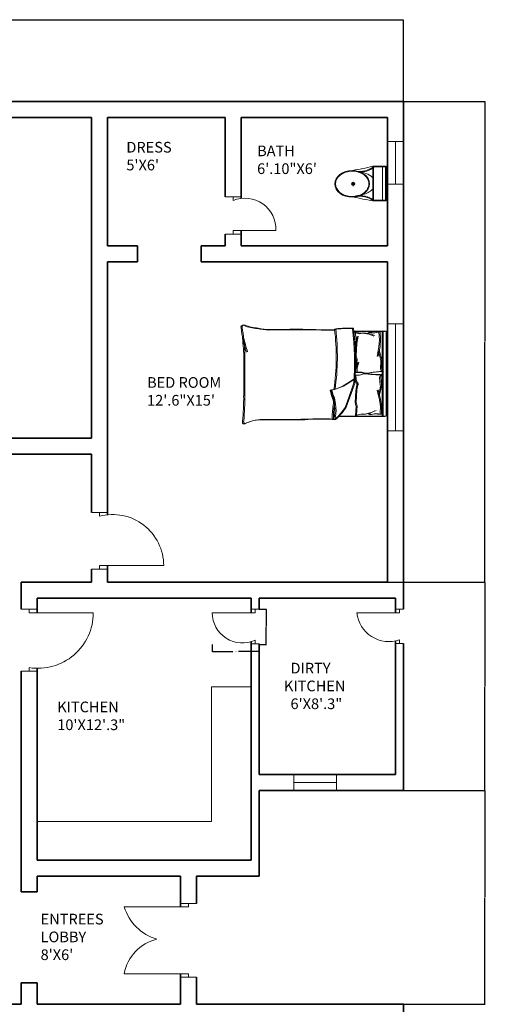
# Model space of a CAD drawing. Units: inches. Extents: x 1824 to 3509, y 619 to 2294.
# Tile 7 of 12: x 2308 to 2569, y 1115 to 1668. Entities that reach past the tile are written whole.
import ezdxf

# ---------------------------------------------------------------- set-up
doc = ezdxf.new("R2010")
doc.units = ezdxf.units.IN
for name, color, linetype, lineweight in [('A-ANNO-DIMS', 2, 'Continuous', 18), ('A-AREA-IDEN', 7, 'Continuous', 18), ('A-DOOR', 3, 'Continuous', 18), ('A-FLOR-FIXT', 9, 'Continuous', 18), ('A-FURN', 8, 'Continuous', 13), ('A-GLAZ', 4, 'Continuous', 18), ('A-WALL', 7, 'Continuous', 35)]:
    doc.layers.add(name, color=color, linetype=linetype, lineweight=lineweight)
doc.styles.get("Standard").update_dxf_attribs({"font": 'arial.ttf'})
doc.dimstyles.get("Standard").update_dxf_attribs({"dimtxt": 0.18, "dimasz": 0.18, "dimexe": 0.18, "dimexo": 0.0625, "dimgap": 0.09, "dimtad": 0, "dimtih": 1, "dimtoh": 1, "dimdec": 4, "dimzin": 0, "dimdsep": 46, "dimtxsty": 'Standard', "dimcen": 0.09, "dimadec": 0, "dimazin": 0, "dimtfac": 1, "dimtdec": 4, "dimtofl": 0, "dimtmove": 0, "dimatfit": 3, "dimfxl": 1, "dimtolj": 1, "dimtzin": 0, "dimarcsym": 0})

# ---------------------------------------------------------------- blocks, each defined once
blk = doc.blocks.new('A$C31115884')
for p, q in [((283, 498), (223, 498)), ((258, 466), (258, 523)), ((0, 200), (0, 0)), ((520, 200), (0, 200)), ((10, 190), (10, 10)), ((510, 190), (10, 190)), ((510, 10), (510, 190)), ((520, 0), (520, 200)), ((510, 54), (0, 54)), ((10, 10), (510, 10)), ((0, 0), (520, 0))]:
    blk.add_line(p, q)
blk.add_circle((256, 496), 23.6)
for centre, radius, start, end in [((2778, -205), 2807, 165.4549, 171.7133), ((-295, 403), 365, 324.2091, 9.3499), ((-295, 403), 375, 324.2091, 9.3499), ((806, 403), 365, 170.6501, 215.7909), ((3237, 905), 2807, 188.2867, 194.5451), ((384, 406), 293, 190.2774, 224.1564), ((139, 406), 293, 315.8436, 2.6563), ((806, 403), 375, 179.2036, 215.7909)]:
    blk.add_arc(centre, radius, start, end)
blk.add_ellipse((256, 510), major_axis=(0, -261), ratio=0.772727)
blk.add_open_spline([(256, 259), (263, 259), (270, 260), (288, 262), (299, 265), (320, 273), (330, 278), (350, 291), (360, 299), (378, 316), (386, 326), (402, 347), (409, 358), (421, 383), (427, 395), (436, 422), (440, 436), (445, 465), (447, 480), (448, 509), (448, 524), (445, 553), (443, 568), (436, 596), (432, 610), (422, 636), (416, 649), (402, 672), (395, 683), (379, 703), (370, 712), (351, 728), (341, 735), (321, 746), (310, 751), (289, 757), (278, 759), (256, 761), (245, 761), (223, 757), (212, 754), (191, 746), (181, 741), (161, 728), (151, 720), (133, 703), (125, 693), (110, 672), (103, 660), (90, 636), (85, 623), (76, 596), (72, 582), (67, 553), (66, 538), (64, 509), (65, 494), (68, 465), (70, 450), (77, 422), (81, 408), (91, 382), (97, 370), (111, 346), (118, 335), (135, 316), (144, 307), (162, 291), (172, 284), (193, 273), (203, 269), (225, 262), (236, 260), (250, 259), (253, 259), (256, 259)], degree=3, knots=[0, 0, 0, 0, 0.110105, 0.110105, 0.285049, 0.285049, 0.459994, 0.459994, 0.634938, 0.634938, 0.809882, 0.809882, 0.984827, 0.984827, 1.159771, 1.159771, 1.334715, 1.334715, 1.50966, 1.50966, 1.684604, 1.684604, 1.859549, 1.859549, 2.034493, 2.034493, 2.209437, 2.209437, 2.384382, 2.384382, 2.559326, 2.559326, 2.73427, 2.73427, 2.909215, 2.909215, 3.084159, 3.084159, 3.259103, 3.259103, 3.434048, 3.434048, 3.608992, 3.608992, 3.783936, 3.783936, 3.958881, 3.958881, 4.133825, 4.133825, 4.30877, 4.30877, 4.483714, 4.483714, 4.658658, 4.658658, 4.833603, 4.833603, 5.008547, 5.008547, 5.183491, 5.183491, 5.358436, 5.358436, 5.53338, 5.53338, 5.708324, 5.708324, 5.883269, 5.883269, 6.058213, 6.058213, 6.233158, 6.233158, 6.283185, 6.283185, 6.283185, 6.283185])
blk = doc.blocks.new('COUNTER-L-PLAN')
for p, q in [((120, 75.53), (97.87, 75.53)), ((97.87, 75.53), (97.87, 75.53)), ((97.87, 75.53), (97.87, 0)), ((97.87, 0), (0, 0))]:
    blk.add_line(p, q)
blk = doc.blocks.new('DOOR-BATH-E-24')
for p, q in [((9, 20.96), (0, 20.96)), ((0, 20.96), (4.5, 20.96)), ((4.5, 20.96), (4.5, 20.96)), ((4.5, 20.96), (4.5, 18.96)), ((0, 0), (9, 0)), ((4.5, 0), (4.5, 2)), ((4.5, 2), (28.5, 2)), ((5.69, 0), (4.5, 0)), ((9, 0), (5.69, 0))]:
    blk.add_line(p, q)
blk.add_arc((11.01, 2.71), 17.51, 357.6736, 111.8197)
blk = doc.blocks.new('DOOR-BED-E-36')
for p, q in [((0, 31.73), (0, 31.73)), ((0, 31.73), (9, 31.73)), ((9, 31.73), (4.5, 31.73)), ((4.5, 31.73), (4.5, 29.73)), ((9, 0), (0, 0)), ((0, 0), (4.5, 0)), ((4.5, 0), (4.5, 2)), ((4.5, 2), (40.5, 2))]:
    blk.add_line(p, q)
blk.add_arc((11.82, 2), 28.68, 0, 104.7949)
blk = doc.blocks.new('DOOR-SIDE-PAIR')
for p, q in [((36, 39.48), (0, 39.48)), ((31.5, 41.48), (40.5, 41.48)), ((40.5, 41.48), (36, 41.48)), ((36, 41.48), (36, 39.48)), ((36, 2), (0, 2)), ((31.5, 0), (40.5, 0)), ((36, 0), (36, 2)), ((40.5, 0), (36, 0))]:
    blk.add_line(p, q)
for centre, radius, start, end in [((26.04, 47.53), 27.26, 197.1823, 253.5499), ((23.91, -2.24), 24.29, 103.3084, 169.936)]:
    blk.add_arc(centre, radius, start, end)
blk = doc.blocks.new('DOOR-SERVICE-EXT-24')
for p, q in [((24, 17.22), (0, 17.22)), ((21.7, 19.22), (26.2, 19.22)), ((26.2, 19.22), (24, 19.22)), ((24, 19.22), (24, 17.22)), ((21.7, 0), (26.2, 0)), ((23.95, 0), (23.95, 2)), ((26.2, 0), (23.95, 0))]:
    blk.add_line(p, q)
blk.add_arc((18.22, 19.44), 18.36, 186.9442, 288.1646)
blk = doc.blocks.new('DOOR-SERVICE-INT-24')
for p, q in [((24, 17.35), (0, 17.35)), ((21.75, 19.35), (26.25, 19.35)), ((24, 19.35), (24, 17.35)), ((21.75, 0), (26.25, 0)), ((24, 0), (24, 2)), ((26.25, 0), (24, 0))]:
    blk.add_line(p, q)
blk.add_arc((16.91, 17.35), 16.91, 180, 294.7994)
blk = doc.blocks.new('DOOR-KITCHEN-36')
for p, q in [((0, 34.79), (9, 34.79)), ((4.5, 34.79), (4.5, 32.79)), ((4.5, 32.79), (40.5, 32.79)), ((4.5, 0), (4.5, 2)), ((0, 0), (9, 0)), ((9, 0), (4.5, 0))]:
    blk.add_line(p, q)
blk.add_arc((9.34, 32.79), 31.16, 261.0709, 0)
blk = doc.blocks.new('BED-DOUBLE-PLAN')
for p, q in [((0, 51.27), (26.61, 51.27)), ((0, 51.27), (26.61, 51.27)), ((0, 3.48), (0, 51.27)), ((0.64, 51.49), (27.25, 51.49)), ((0.64, 51.49), (27.25, 51.49)), ((1.53, 3.48), (1.53, 51.27)), ((1.53, 3.48), (1.53, 51.27)), ((2.17, 3.7), (2.17, 51.49)), ((2.17, 3.7), (2.17, 51.49)), ((2.56, 50.11), (2.46, 44.71)), ((2.56, 50.11), (2.46, 44.71)), ((2.56, 50.11), (5.77, 49.73)), ((2.56, 50.11), (5.77, 49.73)), ((3.2, 50.34), (3.1, 44.94)), ((3.2, 50.34), (3.1, 44.94)), ((3.2, 50.34), (6.41, 49.96)), ((3.2, 50.34), (6.41, 49.96)), ((5.77, 49.73), (8.34, 50.33)), ((5.77, 49.73), (8.34, 50.33)), ((6.41, 49.96), (8.98, 50.56)), ((6.41, 49.96), (8.98, 50.56)), ((11.83, 50.11), (8.26, 49.31)), ((11.83, 50.11), (8.26, 49.31)), ((8.34, 50.33), (9.38, 49.82)), ((8.34, 50.33), (9.38, 49.81)), ((12.47, 50.34), (8.9, 49.54)), ((12.47, 50.34), (8.9, 49.54)), ((8.98, 50.56), (10.02, 50.04)), ((8.98, 50.56), (10.02, 50.04)), ((13.43, 49.92), (11.83, 50.11)), ((13.43, 49.92), (11.83, 50.11)), ((14.07, 50.15), (12.47, 50.34)), ((14.07, 50.15), (12.47, 50.34)), ((16.57, 50.7), (13.43, 49.92)), ((16.57, 50.7), (13.43, 49.92)), ((17.21, 50.93), (14.07, 50.15)), ((17.21, 50.93), (14.07, 50.15)), ((16.17, 45.57), (16.57, 50.7)), ((16.17, 45.57), (16.57, 50.7)), ((16.81, 45.8), (17.21, 50.93)), ((16.81, 45.8), (17.21, 50.93)), ((27.75, 52.87), (24.5, 49.16)), ((27.75, 52.87), (24.5, 49.16)), ((28.39, 53.1), (25.13, 49.39)), ((28.39, 53.1), (25.13, 49.39)), ((29.49, 52.95), (27.75, 52.87, 3.87)), ((29.49, 52.95), (27.75, 52.87, 3.87)), ((28.36, 51.33), (27.75, 52.87)), ((28.36, 51.33), (27.75, 52.87)), ((28.06, 48.23), (28.36, 51.33)), ((28.06, 48.23), (28.36, 51.33)), ((30.13, 53.18), (28.39, 53.1, 3.87)), ((30.13, 53.18), (28.39, 53.1, 3.87)), ((29, 51.56), (28.39, 53.1)), ((29, 51.56), (28.39, 53.1)), ((28.69, 48.46), (29, 51.56)), ((28.69, 48.46), (29, 51.56)), ((2.46, 44.71), (2.54, 45.71)), ((2.46, 44.71), (2.54, 45.71)), ((2.54, 45.71), (3.07, 41.92)), ((2.54, 45.71), (3.07, 41.91)), ((3.1, 44.94), (3.18, 45.94)), ((3.1, 44.94), (3.18, 45.94)), ((3.18, 45.94), (3.71, 42.14)), ((3.18, 45.94), (3.71, 42.14)), ((8.26, 49.31), (5.58, 48.13)), ((8.26, 49.31), (5.58, 48.13)), ((8.9, 49.54), (6.22, 48.36)), ((8.9, 49.54), (6.22, 48.36)), ((16.73, 43.61), (16.17, 45.57)), ((16.73, 43.61), (16.17, 45.57)), ((17.37, 43.84), (16.81, 45.8)), ((17.37, 43.83), (16.81, 45.8)), ((22.33, 46.22), (20.32, 40.64)), ((22.33, 46.22), (20.32, 40.64)), ((22.97, 46.45), (20.96, 40.87)), ((22.97, 46.45), (20.96, 40.87)), ((24.5, 49.16), (22.33, 46.22)), ((24.5, 49.16), (22.33, 46.22)), ((25.13, 49.39), (22.97, 46.45)), ((25.13, 49.39), (22.97, 46.45)), ((28.36, 44.36), (28.06, 48.23)), ((28.36, 44.36), (28.06, 48.23)), ((28.83, 40.95), (28.36, 44.36)), ((28.83, 40.95), (28.36, 44.36)), ((29, 44.59), (28.69, 48.46)), ((29, 44.59), (28.69, 48.46)), ((29.47, 41.18), (29, 44.59)), ((29.47, 41.18), (29, 44.59)), ((3.07, 41.92), (4.42, 36.5)), ((3.07, 41.91), (4.42, 36.5)), ((3.67, 39.2), (3.08, 37.14)), ((3.67, 39.2), (3.08, 37.14)), ((3.71, 42.14), (5.06, 36.72)), ((3.71, 42.14), (5.06, 36.72)), ((4.31, 39.43), (3.72, 37.36)), ((4.31, 39.43), (3.72, 37.36)), ((16.3, 36.6), (16.73, 43.61)), ((16.3, 36.6), (16.73, 43.61)), ((16.93, 36.83), (17.37, 43.84)), ((16.93, 36.82), (17.37, 43.83)), ((20.32, 40.64), (17.38, 32.31)), ((20.32, 40.64), (17.38, 32.31)), ((20.96, 40.87), (18.02, 32.54)), ((20.96, 40.87), (18.02, 32.53)), ((29.76, 38.94), (28.83, 40.95)), ((29.76, 38.94), (28.83, 40.95)), ((30.4, 39.17), (29.47, 41.18)), ((30.4, 39.17), (29.47, 41.18)), ((30.38, 36.46), (29.76, 38.94)), ((30.38, 36.46), (29.76, 38.94)), ((31.02, 36.69), (30.4, 39.17)), ((31.02, 36.69), (30.4, 39.17)), ((79.24, 15.06), (79.24, 39.68)), ((79.24, 15.06), (79.24, 39.68)), ((79.88, 15.29), (79.88, 39.91)), ((79.88, 15.29), (79.88, 39.91)), ((3.08, 37.14), (2.54, 34.21)), ((3.08, 37.14), (2.54, 34.21)), ((2.54, 34.21), (2.56, 33.88)), ((2.54, 34.21), (2.56, 33.88)), ((2.56, 33.88), (2.98, 29.46)), ((2.56, 33.88), (2.98, 29.46)), ((3.72, 37.36), (3.18, 34.43)), ((3.72, 37.36), (3.18, 34.43)), ((3.18, 34.43), (3.2, 34.11)), ((3.18, 34.43), (3.2, 34.11)), ((3.2, 34.11), (3.62, 29.68)), ((3.2, 34.11), (3.62, 29.68)), ((16.74, 30.75), (15.45, 33.82)), ((16.74, 30.75), (15.45, 33.82)), ((15.63, 32.56), (16.3, 36.6)), ((15.63, 32.56), (16.3, 36.6)), ((17.38, 30.98), (16.09, 34.05)), ((17.38, 30.98), (16.09, 34.05)), ((16.27, 32.79), (16.93, 36.83)), ((16.27, 32.79), (16.93, 36.82)), ((17.38, 30.26), (23.88, 34.45)), ((17.38, 30.26), (23.88, 34.45)), ((18.02, 30.49), (24.52, 34.68)), ((18.02, 30.49), (24.52, 34.68)), ((23.88, 34.45), (28.36, 36.15)), ((23.88, 34.45), (28.36, 36.15)), ((24.52, 34.68), (29, 36.38)), ((24.52, 34.68), (29, 36.38)), ((28.36, 36.15), (30.38, 36.46)), ((28.36, 36.15), (30.38, 36.46)), ((29, 36.38), (31.02, 36.69)), ((29, 36.38), (31.02, 36.69)), ((2.98, 29.46), (2.49, 27.98)), ((2.98, 29.46), (2.49, 27.98)), ((2.49, 27.98), (7.87, 27.73)), ((2.49, 27.98), (7.87, 27.73)), ((3.62, 29.68), (3.13, 28.21)), ((3.62, 29.68), (3.13, 28.21)), ((3.13, 28.21), (8.51, 27.96)), ((3.13, 28.21), (8.51, 27.96)), ((7.87, 27.73), (11.08, 27.36)), ((7.87, 27.73), (11.08, 27.36)), ((8.51, 27.96), (11.72, 27.58)), ((8.51, 27.96), (11.72, 27.58)), ((11.72, 27.58), (13.02, 27.67)), ((11.72, 27.58), (13.02, 27.66)), ((12.38, 27.44), (14.22, 28.13)), ((12.38, 27.44), (14.22, 28.13)), ((13.02, 27.67), (14.86, 28.36)), ((13.02, 27.66), (14.86, 28.36)), ((14.22, 28.13), (16.89, 28.3)), ((14.22, 28.13), (16.89, 28.3)), ((14.86, 28.36), (17.53, 28.53)), ((14.86, 28.36), (17.53, 28.53)), ((16.89, 28.3), (16.74, 30.75)), ((16.89, 28.3), (16.74, 30.75)), ((17.53, 28.53), (17.38, 30.98)), ((17.53, 28.53), (17.38, 30.98)), ((1.87, 25.98), (7.22, 26.56)), ((1.87, 25.98), (7.22, 26.56)), ((2.45, 24.54), (1.87, 25.98)), ((2.45, 24.54), (1.87, 25.98)), ((2.3, 20.09), (2.45, 24.54)), ((2.3, 20.09), (2.45, 24.54)), ((2.51, 26.21), (7.86, 26.79)), ((2.51, 26.21), (7.86, 26.79)), ((3.09, 24.77), (2.51, 26.21)), ((3.09, 24.77), (2.51, 26.21)), ((2.94, 20.32), (3.09, 24.77)), ((2.94, 20.32), (3.09, 24.77)), ((7.22, 26.56), (10.4, 27.14)), ((7.22, 26.56), (10.4, 27.14)), ((7.86, 26.79), (11.04, 27.37)), ((7.86, 26.79), (11.04, 27.37)), ((10.4, 27.14), (11.7, 27.14)), ((10.4, 27.14), (11.7, 27.14)), ((11.04, 27.37), (12.34, 27.37)), ((11.04, 27.37), (12.34, 27.37)), ((11.08, 27.36), (12.38, 27.44)), ((11.08, 27.36), (12.38, 27.44)), ((11.7, 27.14), (13.58, 26.56)), ((11.7, 27.14), (13.58, 26.56)), ((12.34, 27.37), (14.22, 26.79)), ((12.34, 27.37), (14.22, 26.79)), ((13.58, 26.56), (16.26, 26.56)), ((13.58, 26.56), (16.26, 26.56)), ((14.22, 26.79), (16.9, 26.79)), ((14.22, 26.79), (16.9, 26.79)), ((16.26, 24.1), (15.17, 20.96)), ((16.26, 24.1), (15.17, 20.96)), ((16.9, 24.33), (15.81, 21.19)), ((16.9, 24.33), (15.81, 21.19)), ((16.17, 19.38), (16.57, 24.52)), ((16.17, 19.38), (16.57, 24.52)), ((16.26, 26.56), (16.26, 24.1)), ((16.26, 26.56), (16.26, 24.1)), ((16.81, 19.61), (17.21, 24.74)), ((16.81, 19.61), (17.21, 24.74)), ((16.9, 26.79), (16.9, 24.33)), ((16.9, 26.79), (16.9, 24.33)), ((2.3, 19.77), (2.3, 20.09)), ((2.3, 19.77), (2.3, 20.09)), ((3.03, 16.88), (2.3, 19.77)), ((3.03, 16.88), (2.3, 19.77)), ((2.94, 20), (2.94, 20.32)), ((2.94, 20), (2.94, 20.32)), ((3.67, 17.11), (2.94, 20)), ((3.67, 17.11), (2.94, 20)), ((3.75, 14.86), (3.03, 16.88)), ((3.75, 14.86), (3.03, 16.88)), ((3.32, 12.11), (4.33, 17.6)), ((3.32, 12.11), (4.33, 17.6)), ((4.39, 15.08), (3.67, 17.11)), ((4.39, 15.08), (3.67, 17.11)), ((3.96, 12.34), (4.97, 17.83)), ((3.96, 12.34), (4.97, 17.83)), ((16.73, 17.42), (16.17, 19.38)), ((16.73, 17.42), (16.17, 19.38)), ((16.3, 10.41), (16.73, 17.42)), ((16.3, 10.41), (16.73, 17.42)), ((17.37, 17.65), (16.81, 19.61)), ((17.37, 17.65), (16.81, 19.61)), ((16.93, 10.64), (17.37, 17.65)), ((16.93, 10.64), (17.37, 17.65)), ((3.03, 8.29), (3.32, 12.11)), ((3.03, 8.29), (3.32, 12.11)), ((3.67, 8.51), (3.96, 12.34)), ((3.67, 8.51), (3.96, 12.34)), ((3.01, 8.18), (3.03, 8.29)), ((3.01, 8.18), (3.03, 8.29)), ((3.34, 3.9), (3.01, 8.18)), ((3.34, 3.9), (3.01, 8.18)), ((3.65, 8.41), (3.67, 8.51)), ((3.65, 8.41), (3.67, 8.51)), ((3.98, 4.13), (3.65, 8.41)), ((3.98, 4.13), (3.65, 8.41)), ((8.95, 5.05), (6.21, 6.06)), ((8.95, 5.05), (6.21, 6.06)), ((9.59, 5.28), (6.85, 6.29)), ((9.59, 5.28), (6.85, 6.29)), ((15.63, 6.38), (16.3, 10.41)), ((15.63, 6.38), (16.3, 10.41)), ((16.27, 6.61), (16.93, 10.64)), ((16.27, 6.61), (16.93, 10.64)), ((16.3, 10.41), (16.62, 9.28)), ((16.3, 10.41), (16.62, 9.28)), ((16.62, 9.28), (17.34, 4.18)), ((16.62, 9.28), (17.34, 4.18)), ((16.93, 10.64), (17.26, 9.51)), ((16.93, 10.64), (17.26, 9.51)), ((17.26, 9.51), (17.98, 4.41)), ((17.26, 9.51), (17.98, 4.41)), ((18.11, 3.48), (0, 3.48)), ((18.11, 3.48), (0, 3.48)), ((18.75, 3.7), (0.64, 3.7)), ((18.75, 3.7), (0.64, 3.7)), ((3.32, 3.9), (6.5, 4.47)), ((3.32, 3.9), (6.5, 4.47)), ((3.96, 4.12), (7.14, 4.7)), ((3.96, 4.12), (7.14, 4.7)), ((6.5, 4.47), (9.1, 4.04)), ((6.5, 4.47), (9.1, 4.04)), ((7.14, 4.7), (9.74, 4.27)), ((7.14, 4.7), (9.74, 4.27)), ((12.57, 4.47), (8.95, 5.05)), ((12.57, 4.47), (8.95, 5.05)), ((9.1, 4.04), (10.11, 4.62)), ((9.1, 4.04), (10.11, 4.62)), ((13.21, 4.7), (9.59, 5.28)), ((13.21, 4.7), (9.59, 5.28)), ((9.74, 4.27), (10.75, 4.85)), ((9.74, 4.27), (10.75, 4.85)), ((14.16, 4.76), (12.57, 4.47)), ((14.16, 4.76), (12.57, 4.47)), ((14.8, 4.99), (13.21, 4.7)), ((14.8, 4.99), (13.21, 4.7)), ((17.34, 4.18), (14.16, 4.76)), ((17.34, 4.18), (14.16, 4.76)), ((17.98, 4.41), (14.8, 4.99)), ((17.98, 4.41), (14.8, 4.99))]:
    blk.add_line(p, q)
for centre, radius, start, end in [((68.67, 76.16), 23.07, 267.4714, 296.4681), ((68.67, 76.16), 23.07, 267.4714, 296.4681), ((69.31, 76.39), 23.07, 267.4714, 296.4681), ((69.31, 76.39), 23.07, 267.4714, 296.4681), ((78.87, 54.41), 1.1, 332.6588, 86.02), ((78.87, 54.41), 1.1, 332.6588, 86.02), ((79.51, 54.64), 1.1, 332.6588, 86.02), ((79.51, 54.64), 1.1, 332.6588, 86.02), ((-6.66, 51.33), 36.18, 349.8763, 2.5657), ((-6.66, 51.33), 36.18, 349.8763, 2.5657), ((36.32, 182.27), 129.5, 266.9791, 273.8365), ((36.32, 182.27), 129.5, 266.9791, 273.8365), ((-6.02, 51.56), 36.18, 349.8763, 2.5657), ((-6.02, 51.56), 36.18, 349.8763, 2.5657), ((36.95, 182.49), 129.5, 266.9791, 273.8365), ((36.95, 182.49), 129.5, 266.9791, 273.8365), ((67.82, -4508.74), 4561.86, 90.00217, 90.28689), ((67.82, -4508.74), 4561.86, 90.00217, 90.28689), ((68.46, -4508.51), 4561.86, 90.00217, 90.28689), ((68.46, -4508.51), 4561.86, 90.00217, 90.28689), ((212.28, 41.15), 133.04, 174.4998, 180.6351), ((212.28, 41.15), 133.04, 174.4998, 180.6351), ((212.92, 41.38), 133.04, 174.4998, 180.6351), ((212.92, 41.38), 133.04, 174.4998, 180.6351), ((35.07, 43.74), 6.22, 168.6608, 203.7384), ((35.07, 43.74), 6.22, 168.6608, 203.7384), ((35.71, 43.97), 6.22, 168.6608, 203.7384), ((35.71, 43.97), 6.22, 168.6608, 203.7384), ((1.48, 31.15), 29.65, 10.6617, 19.8806), ((1.48, 31.15), 29.65, 10.6617, 19.8806), ((2.12, 31.38), 29.65, 10.6617, 19.8806), ((2.12, 31.38), 29.65, 10.6617, 19.8806), ((156.32, 17.76), 129.02, 171.7845, 186.9006), ((156.32, 17.76), 129.02, 171.7845, 186.9006), ((156.96, 17.98), 129.02, 171.7845, 186.9006), ((156.96, 17.98), 129.02, 171.7845, 186.9006), ((30.44, 36.64), 0.185, 250.2464, 1.1377), ((30.44, 36.64), 0.185, 250.2464, 1.1377), ((31.08, 36.87), 0.185, 250.2464, 1.1377), ((31.08, 36.87), 0.185, 250.2464, 1.1377), ((182.05, 21.36), 164.97, 176.0865, 186.7821), ((182.05, 21.36), 164.97, 176.0865, 186.7821), ((182.69, 21.59), 164.97, 176.0865, 186.7821), ((182.69, 21.59), 164.97, 176.0865, 186.7821), ((-23.71, -17.22), 106.46, 13.3832, 17.7053), ((-23.71, -17.22), 106.46, 13.3832, 17.7053), ((-23.07, -16.99), 106.46, 13.3832, 17.7053), ((-23.07, -16.99), 106.46, 13.3832, 17.7053), ((200.84, 21.43), 121.76, 182.9958, 189.4091), ((200.84, 21.43), 121.76, 182.9958, 189.4091), ((201.48, 21.66), 121.76, 182.9958, 189.4091), ((201.48, 21.66), 121.76, 182.9958, 189.4091), ((20.1, 85.16), 83.31, 268.7218, 275.604), ((20.1, 85.16), 83.31, 268.7218, 275.604), ((20.74, 85.39), 83.31, 268.7218, 275.604), ((20.74, 85.39), 83.31, 268.7218, 275.604), ((31.17, -167.31), 170.11, 88.4762, 91.0082), ((31.17, -167.31), 170.11, 88.4762, 91.0082), ((31.81, -167.08), 170.11, 88.4762, 91.0082), ((31.81, -167.08), 170.11, 88.4762, 91.0082), ((50.61, 484.82), 482.31, 268.2277, 271.7185), ((50.61, 484.82), 482.31, 268.2277, 271.7185), ((51.25, 485.05), 482.31, 268.2277, 271.7185), ((51.25, 485.05), 482.31, 268.2277, 271.7185), ((64.52, -26.9), 29.63, 76.0648, 88.9113), ((64.52, -26.9), 29.63, 76.0648, 88.9113), ((65.15, -26.67), 29.63, 76.0648, 88.9113), ((65.15, -26.67), 29.63, 76.0648, 88.9113), ((70.28, -21.66), 23.56, 67.9751, 86.652), ((70.28, -21.66), 23.56, 67.9751, 86.652), ((70.91, -21.43), 23.56, 67.9751, 86.652), ((70.91, -21.43), 23.56, 67.9751, 86.652), ((79.72, 1.09), 1.09, 236.1736, 23.4781), ((79.72, 1.09), 1.09, 236.1736, 23.4781), ((80.36, 1.32), 1.09, 236.1736, 23.4781), ((80.36, 1.32), 1.09, 236.1736, 23.4781)]:
    blk.add_arc(centre, radius, start, end)
blk = doc.blocks.new('WIN-24')
for p, q in [((0, 0), (0, 9)), ((0, 9), (0, 4.5)), ((24, 0), (24, 9)), ((0, 4.5), (24, 4.5)), ((24, 4.5), (24, 0))]:
    blk.add_line(p, q)
blk = doc.blocks.new('WIN-60')
for p, q in [((0, 9), (0, 0)), ((60, 4.5), (60, 9)), ((60, 9), (60, 0)), ((0, 0), (0, 4.5)), ((0, 4.5), (60, 4.5))]:
    blk.add_line(p, q)
blk = doc.blocks.new('*D70')
at = {"layer": 'A-ANNO-DIMS', "color": 0, "lineweight": -2, "transparency": 16777216}
for p, q in [((2415.84, 1317.1), (2415.84, 1313.04)), ((2442.09, 1317.1), (2442.09, 1313.04)), ((2416.02, 1313.22), (2427.44, 1313.22)), ((2441.91, 1313.22), (2430.49, 1313.22))]:
    blk.add_line(p, q, dxfattribs=at)
at = {"layer": 'A-ANNO-DIMS', "color": 0, "transparency": 16777216}
for points in [[(2416.02, 1313.25), (2416.02, 1313.19), (2415.84, 1313.22)], [(2441.91, 1313.25), (2441.91, 1313.19), (2442.09, 1313.22)]]:
    blk.add_solid(points, dxfattribs=at)
at = {"layer": 'Defpoints', "color": 0, "transparency": 16777216}
for p in [(2415.84, 1317.16), (2442.09, 1317.16), (2442.09, 1313.22)]:
    blk.add_point(p, dxfattribs=at)
at = {"layer": 'A-ANNO-DIMS', "color": 0, "transparency": 16777216, "insert": (2428.96, 1313.22), "char_height": 0.18, "attachment_point": 5}
blk.add_mtext('\\A1;SERVICE DOOR 26 TYP.', dxfattribs=at)
blk = doc.blocks.new('*D71')
at = {"layer": 'A-ANNO-DIMS', "color": 0, "lineweight": -2, "transparency": 16777216}
for p, q in [((2442.15, 1336.93), (2446.21, 1336.93)), ((2446.03, 1336.75), (2446.03, 1327.23)), ((2446.03, 1317.34), (2446.03, 1326.86)), ((2442.15, 1317.16), (2446.21, 1317.16))]:
    blk.add_line(p, q, dxfattribs=at)
at = {"layer": 'A-ANNO-DIMS', "color": 0, "transparency": 16777216}
for points in [[(2446, 1336.75), (2446.06, 1336.75), (2446.03, 1336.93)], [(2446, 1317.34), (2446.06, 1317.34), (2446.03, 1317.16)]]:
    blk.add_solid(points, dxfattribs=at)
at = {"layer": 'Defpoints', "color": 0, "transparency": 16777216}
for p in [(2442.09, 1336.93), (2446.03, 1336.93), (2442.09, 1317.16)]:
    blk.add_point(p, dxfattribs=at)
at = {"layer": 'A-ANNO-DIMS', "color": 0, "transparency": 16777216, "insert": (2446.03, 1327.05), "char_height": 0.18, "attachment_point": 5}
blk.add_mtext('\\A1;20 TYP.', dxfattribs=at)
blk = doc.blocks.new('*D94')
at = {"layer": 'A-ANNO-DIMS', "color": 0, "lineweight": -2, "transparency": 16777216}
for p, q in [((1949.09, 1049.16), (1949.09, 1668.03)), ((1949.27, 1667.85), (2235.8, 1667.85)), ((2522.91, 1667.85), (2236.38, 1667.85)), ((2523.09, 1622.16), (2523.09, 1668.03))]:
    blk.add_line(p, q, dxfattribs=at)
at = {"layer": 'A-ANNO-DIMS', "color": 0, "transparency": 16777216}
for points in [[(1949.27, 1667.88), (1949.27, 1667.82), (1949.09, 1667.85)], [(2522.91, 1667.88), (2522.91, 1667.82), (2523.09, 1667.85)]]:
    blk.add_solid(points, dxfattribs=at)
at = {"layer": 'Defpoints', "color": 0, "transparency": 16777216}
for p in [(2523.09, 1667.85), (2523.09, 1622.1), (1949.09, 1049.1)]:
    blk.add_point(p, dxfattribs=at)
at = {"layer": 'A-ANNO-DIMS', "color": 0, "transparency": 16777216, "insert": (2236.09, 1667.85), "char_height": 0.18, "attachment_point": 5}
blk.add_mtext('\\A1;574', dxfattribs=at)
blk = doc.blocks.new('*D98')
at = {"layer": 'A-ANNO-DIMS', "color": 0, "lineweight": -2, "transparency": 16777216}
for p, q in [((2523.15, 1235.1), (2569.02, 1235.1)), ((2568.84, 1234.92), (2568.84, 1175.28)), ((2568.84, 1115.28), (2568.84, 1174.92)), ((2523.15, 1115.1), (2569.02, 1115.1))]:
    blk.add_line(p, q, dxfattribs=at)
at = {"layer": 'A-ANNO-DIMS', "color": 0, "transparency": 16777216}
for points in [[(2568.81, 1234.92), (2568.87, 1234.92), (2568.84, 1235.1)], [(2568.81, 1115.28), (2568.87, 1115.28), (2568.84, 1115.1)]]:
    blk.add_solid(points, dxfattribs=at)
at = {"layer": 'Defpoints', "color": 0, "transparency": 16777216}
for p in [(2523.09, 1235.1), (2568.84, 1235.1), (2523.09, 1115.1)]:
    blk.add_point(p, dxfattribs=at)
at = {"layer": 'A-ANNO-DIMS', "color": 0, "transparency": 16777216, "insert": (2568.84, 1175.1), "char_height": 0.18, "attachment_point": 5}
blk.add_mtext('\\A1;120', dxfattribs=at)
blk = doc.blocks.new('*D99')
at = {"layer": 'A-ANNO-DIMS', "color": 0, "lineweight": -2, "transparency": 16777216}
for p, q in [((2514.15, 1352.1), (2569.02, 1352.1)), ((2568.84, 1351.92), (2568.84, 1293.78)), ((2568.84, 1235.28), (2568.84, 1293.42)), ((2523.15, 1235.1), (2569.02, 1235.1))]:
    blk.add_line(p, q, dxfattribs=at)
at = {"layer": 'A-ANNO-DIMS', "color": 0, "transparency": 16777216}
for points in [[(2568.81, 1351.92), (2568.87, 1351.92), (2568.84, 1352.1)], [(2568.81, 1235.28), (2568.87, 1235.28), (2568.84, 1235.1)]]:
    blk.add_solid(points, dxfattribs=at)
at = {"layer": 'Defpoints', "color": 0, "transparency": 16777216}
for p in [(2514.09, 1352.1), (2568.84, 1352.1), (2523.09, 1235.1)]:
    blk.add_point(p, dxfattribs=at)
at = {"layer": 'A-ANNO-DIMS', "color": 0, "transparency": 16777216, "insert": (2568.84, 1293.6), "char_height": 0.18, "attachment_point": 5}
blk.add_mtext('\\A1;117', dxfattribs=at)
blk = doc.blocks.new('*D100')
at = {"layer": 'A-ANNO-DIMS', "color": 0, "lineweight": -2, "transparency": 16777216}
for p, q in [((2523.15, 1622.1), (2569.02, 1622.1)), ((2568.84, 1621.92), (2568.84, 1487.28)), ((2568.84, 1352.28), (2568.84, 1486.92)), ((2514.15, 1352.1), (2569.02, 1352.1))]:
    blk.add_line(p, q, dxfattribs=at)
at = {"layer": 'A-ANNO-DIMS', "color": 0, "transparency": 16777216}
for points in [[(2568.81, 1621.92), (2568.87, 1621.92), (2568.84, 1622.1)], [(2568.81, 1352.28), (2568.87, 1352.28), (2568.84, 1352.1)]]:
    blk.add_solid(points, dxfattribs=at)
at = {"layer": 'Defpoints', "color": 0, "transparency": 16777216}
for p in [(2523.09, 1622.1), (2568.84, 1622.1), (2514.09, 1352.1)]:
    blk.add_point(p, dxfattribs=at)
at = {"layer": 'A-ANNO-DIMS', "color": 0, "transparency": 16777216, "insert": (2568.84, 1487.1), "char_height": 0.18, "attachment_point": 5}
blk.add_mtext('\\A1;270', dxfattribs=at)

msp = doc.modelspace()

# ---------------------------------------------------------------- linework, layer by layer
at = {"layer": 'A-GLAZ'}
msp.add_line((2523.0899, 1599.654), (2523.0899, 1599.654), dxfattribs=at)
at = {"layer": 'A-WALL'}
for p, q in [((2006.0899, 1622.1012), (2523.0899, 1622.1012)), ((2523.0899, 1622.1012), (2523.0899, 1336.9292)), ((2192.0899, 1613.1012), (2348.0899, 1613.1012)), ((2348.0899, 1613.1012), (2348.0899, 1433.1012)), ((2357.0899, 1613.1012), (2357.0899, 1541.1012)), ((2357.0899, 1613.1012), (2423.0899, 1613.1012)), ((2423.0899, 1613.1012), (2423.0899, 1568.5597)), ((2432.0899, 1613.1012), (2432.0899, 1567.6985)), ((2432.0899, 1613.1012), (2514.0899, 1613.1012)), ((2514.0899, 1613.1012), (2514.0899, 1541.1012)), ((2432.0899, 1549.5961), (2432.0899, 1541.1012)), ((2423.0899, 1547.5961), (2423.0899, 1541.1012)), ((2357.0899, 1541.1012), (2373.9772, 1541.1012)), ((2373.9772, 1541.1012), (2373.9772, 1532.1012)), ((2409.6371, 1541.1012), (2409.6371, 1532.1012)), ((2409.6371, 1541.1012), (2423.0899, 1541.1012)), ((2432.0899, 1541.1012), (2514.0899, 1541.1012)), ((2357.0899, 1532.1012), (2373.9772, 1532.1012)), ((2357.0899, 1532.1012), (2357.0899, 1390.0103)), ((2409.6371, 1532.1012), (2514.0899, 1532.1012)), ((2514.0899, 1532.1012), (2514.0899, 1352.1012)), ((2235.3516, 1433.1012), (2348.0899, 1433.1012)), ((2237.6334, 1424.1012), (2348.0899, 1424.1012)), ((2348.0899, 1424.1012), (2348.0899, 1391.1988)), ((2357.0899, 1361.4725), (2357.0899, 1352.1012)), ((2348.0899, 1359.4725), (2348.0899, 1352.1012)), ((2308.5899, 1343.1012), (2308.5899, 1352.1012)), ((2308.5899, 1352.1012), (2348.0899, 1352.1012)), ((2357.0899, 1352.1012), (2514.0899, 1352.1012)), ((2308.5899, 1343.1012), (2308.5899, 1336.9292)), ((2317.5899, 1343.1012), (2317.5899, 1334.9292)), ((2357.0899, 1343.1012), (2317.5899, 1343.1012)), ((2357.0899, 1343.1012), (2437.5899, 1343.1012)), ((2437.5899, 1343.1012), (2437.5899, 1334.9292)), ((2442.0899, 1343.1012), (2442.0899, 1336.9292)), ((2442.0899, 1343.1012), (2514.0899, 1343.1012)), ((2514.0899, 1343.1012), (2518.5899, 1343.1012)), ((2518.5899, 1343.1012), (2518.5899, 1334.9292)), ((2437.5899, 1318.7293), (2437.5899, 1196.1012)), ((2442.0899, 1317.5804), (2442.0899, 1244.1012)), ((2518.5899, 1319.1219), (2518.5899, 1244.1012)), ((2523.0899, 1317.7052), (2523.0899, 1235.1012)), ((2308.5899, 1302.1437), (2308.5899, 1178.3005)), ((2317.5899, 1303.7679), (2317.5899, 1196.1012)), ((2442.0899, 1244.1012), (2518.5899, 1244.1012)), ((2442.0899, 1235.1012), (2514.0899, 1235.1012)), ((2442.0899, 1235.1012), (2442.0899, 1187.1012)), ((2514.0899, 1235.1012), (2523.0899, 1235.1012)), ((2357.0899, 1196.1012), (2317.5899, 1196.1012)), ((2357.0899, 1196.1012), (2437.5899, 1196.1012)), ((2357.0899, 1187.1012), (2317.5899, 1187.1012)), ((2317.5899, 1187.1012), (2317.5899, 1178.3005)), ((2357.0899, 1187.1012), (2397.9516, 1187.1012)), ((2397.9516, 1187.1012), (2397.9516, 1169.754)), ((2406.9516, 1171.754), (2406.9516, 1187.1012)), ((2406.9516, 1187.1012), (2442.0899, 1187.1012)), ((2317.5899, 1178.3005), (2308.5899, 1178.3005)), ((2397.9516, 1132.2745), (2397.9516, 1115.1012)), ((2406.9516, 1115.1012), (2406.9516, 1130.2745)), ((2317.5899, 1127.2043), (2308.5899, 1127.2043)), ((2308.5899, 1127.2043), (2308.5899, 1115.1012)), ((2317.5899, 1127.2043), (2317.5899, 1115.1012)), ((2308.5899, 1115.1012), (2273.8478, 1115.1012)), ((2397.9516, 1115.1012), (2317.5899, 1115.1012)), ((2357.0899, 1115.1012), (2397.9516, 1115.1012)), ((2406.9516, 1115.1012), (2514.0899, 1115.1012)), ((2514.0899, 1115.1012), (2523.0899, 1115.1012)), ((2523.0899, 1115.1012), (2523.0899, 818.1012))]:
    msp.add_line(p, q, dxfattribs=at)

# ---------------------------------------------------------------- block references
at = {"layer": 'A-DOOR'}
for name, p in [('DOOR-BATH-E-24', (2423.09, 1547.596)), ('DOOR-BED-E-36', (2348.09, 1359.472)), ('DOOR-KITCHEN-36', (2308.59, 1302.144)), ('DOOR-SERVICE-INT-24', (2415.84, 1317.58)), ('DOOR-SERVICE-EXT-24', (2496.893, 1317.705)), ('DOOR-SIDE-PAIR', (2366.452, 1130.274))]:
    msp.add_blockref(name, p, dxfattribs=at)
at = {"layer": 'A-FLOR-FIXT', "xscale": 0.0372717239612423, "yscale": 0.0372717239612423, "zscale": 0.0372717239612423, "rotation": 90.2893490319937}
msp.add_blockref('A$C31115884', (2513.4288, 1566.3918), dxfattribs=at)
at = {"layer": 'A-FLOR-FIXT'}
msp.add_blockref('COUNTER-L-PLAN', (2317.59, 1217.851), dxfattribs=at)
at = {"layer": 'A-FURN', "rotation": 180}
msp.add_blockref('BED-DOUBLE-PLAN', (2513.3429, 1496.6876), dxfattribs=at)
msp.add_blockref('BED-DOUBLE-PLAN', (2513.3429, 1496.6876), dxfattribs=at)
at = {"layer": 'A-GLAZ', "rotation": 270}
msp.add_blockref('WIN-24', (2514.0897, 1599.6544), dxfattribs=at)
at = {"layer": 'A-GLAZ', "extrusion": (0, 0, -1), "zscale": -1}
for name, p, rotation in [('WIN-60', (-2514.0897, 1437.2381), 90), ('WIN-24', (-2461.5652, 1244.1013), 180)]:
    msp.add_blockref(name, p, dxfattribs=dict(at, rotation=rotation))

# ---------------------------------------------------------------- texts
at = {"layer": 'A-AREA-IDEN', "char_height": 6, "attachment_point": 1}
for s, width, insert in [("DRESS\\P5'X6'", 46.699478, (2367.6304, 1599.4136)), ('BATH\\P6\'.10"X6\'', 59.011464, (2440.9915, 1597.3766)), ('BED ROOM\\P12\'.6"X15\'', 121.482018, (2379.2447, 1467.3102)), ('  DIRTY\\PKITCHEN\\P  6\'X8\'.3"', 51.430052, (2456.0649, 1306.8812)), ('KITCHEN\\P10\'X12\'.3"', 70.975091, (2328.8457, 1285.0876))]:
    msp.add_mtext_dynamic_manual_height_columns(s, width=width, gutter_width=12.5, heights=[0], dxfattribs=dict(at, insert=insert))
at = {"layer": 'A-AREA-IDEN', "insert": (2319.505, 1165.9525), "char_height": 6, "width": 67.257605, "attachment_point": 1}
msp.add_mtext("ENTREES\\P  LOBBY\\P   8'X6'", dxfattribs=at)

# ---------------------------------------------------------------- dimensions: what is measured, and where the dimension line sits
at = {"layer": 'A-ANNO-DIMS'}
dim = msp.add_linear_dim(base=(2523.0899, 1667.8512), p1=(1949.0899, 1049.1012), p2=(2523.0899, 1622.1012), dimstyle='Standard', override={"dimdec": 0, "dimlfac": 1, "dimrnd": 0, "dimzin": 0, "dimdsep": 46, "dimlunit": 2}, dxfattribs=at)
dim.commit()
dim.dimension.update_dxf_attribs({"geometry": '*D94', "text_midpoint": (2236.0899, 1667.8512)})
for base, p1, p2, picture, middle in [((2568.8399, 1622.1012), (2514.0899, 1352.1012), (2523.0899, 1622.1012), '*D100', (2568.8399, 1487.1012)), ((2568.8399, 1352.1012), (2523.0899, 1235.1012), (2514.0899, 1352.1012), '*D99', (2568.8399, 1293.6012)), ((2568.8399, 1235.1012), (2523.0899, 1115.1012), (2523.0899, 1235.1012), '*D98', (2568.8399, 1175.1012))]:
    dim = msp.add_linear_dim(base=base, p1=p1, p2=p2, angle=90, dimstyle='Standard', override={"dimdec": 0, "dimlfac": 1, "dimrnd": 0, "dimzin": 0, "dimdsep": 46, "dimlunit": 2}, dxfattribs=at)
    dim.commit()
    dim.dimension.update_dxf_attribs({"geometry": picture, "text_midpoint": middle})
dim = msp.add_linear_dim(base=(2446.0274, 1336.9292), p1=(2442.0899, 1317.1613), p2=(2442.0899, 1336.9292), angle=90, text='<> TYP.', dimstyle='Standard', override={"dimdec": 0, "dimlfac": 1, "dimrnd": 0, "dimzin": 0, "dimdsep": 46, "dimlunit": 2}, dxfattribs=at)
dim.commit()
dim.dimension.update_dxf_attribs({"geometry": '*D71', "text_midpoint": (2446.0274, 1327.0453)})
dim = msp.add_linear_dim(base=(2442.0899, 1313.2238), p1=(2415.8399, 1317.1613), p2=(2442.0899, 1317.1613), text='SERVICE DOOR <> TYP.', dimstyle='Standard', override={"dimdec": 0, "dimlfac": 1, "dimrnd": 0, "dimzin": 0, "dimdsep": 46, "dimlunit": 2}, dxfattribs=at)
dim.commit()
dim.dimension.update_dxf_attribs({"geometry": '*D70', "text_midpoint": (2428.9649, 1313.2238)})

doc.saveas('drawing.dxf')
